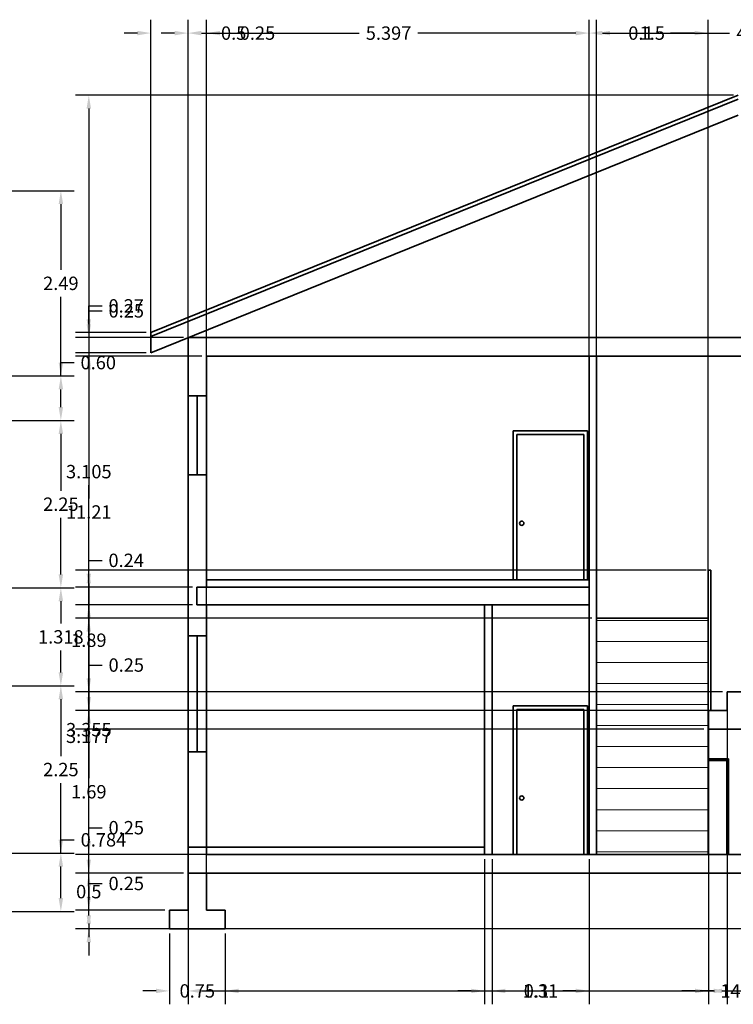
# Model space of a CAD drawing. Units: metres. Extents: x 14054 to 28215, y 4175 to 8383.
# Tile 5 of 6: x 14096.96 to 14106.56, y 4179.48 to 4192.72. Entities that reach past the tile are written whole.
import ezdxf

# ---------------------------------------------------------------- set-up
doc = ezdxf.new("R2010")
doc.units = ezdxf.units.M
for name, color, linetype, lineweight in [('A-ANNO-DIMS', 2, 'Continuous', 18), ('A-ANNO-NPLT', 9, 'Continuous', 13), ('A-SECT', 1, 'Continuous', 35), ('A-WALL-PATT', 8, 'Continuous', 13)]:
    doc.layers.add(name, color=color, linetype=linetype, lineweight=lineweight)
doc.styles.get("Standard").update_dxf_attribs({"font": 'arial.ttf'})
doc.dimstyles.get("Standard").update_dxf_attribs({"dimtxt": 0.18, "dimasz": 0.18, "dimexe": 0.18, "dimexo": 0.0625, "dimgap": 0.09, "dimtad": 0, "dimtih": 1, "dimtoh": 1, "dimdec": 4, "dimzin": 0, "dimdsep": 46, "dimtxsty": 'Standard', "dimcen": 0.09, "dimadec": 0, "dimazin": 0, "dimtfac": 1, "dimtdec": 4, "dimtofl": 0, "dimtmove": 0, "dimatfit": 3, "dimfxl": 1, "dimtolj": 1, "dimtzin": 0, "dimarcsym": 0})

# ---------------------------------------------------------------- blocks, each defined once
blk = doc.blocks.new('*D23')
at = {"layer": 'A-ANNO-DIMS', "color": 0, "lineweight": -2, "transparency": 16777216}
for p, q in [((14097.511, 4181.511), (14097.511, 4181.691)), ((14097.511, 4181.691), (14097.691, 4181.691)), ((14092.904, 4181.511), (14097.691, 4181.511)), ((14097.511, 4180.908), (14097.511, 4181.331)), ((14094.951, 4180.728), (14097.691, 4180.728))]:
    blk.add_line(p, q, dxfattribs=at)
at = {"layer": 'A-ANNO-DIMS', "color": 0, "transparency": 16777216}
for points in [[(14097.481, 4181.331), (14097.541, 4181.331), (14097.511, 4181.511)], [(14097.481, 4180.908), (14097.541, 4180.908), (14097.511, 4180.728)]]:
    blk.add_solid(points, dxfattribs=at)
at = {"layer": 'Defpoints', "color": 0, "transparency": 16777216}
for p in [(14092.842, 4181.511), (14097.511, 4181.511), (14094.888, 4180.728)]:
    blk.add_point(p, dxfattribs=at)
at = {"layer": 'A-ANNO-DIMS', "color": 0, "transparency": 16777216, "insert": (14098.084, 4181.691), "char_height": 0.18, "attachment_point": 5}
blk.add_mtext('\\A1;0.784', dxfattribs=at)
blk = doc.blocks.new('*D24')
at = {"layer": 'A-ANNO-DIMS', "color": 0, "lineweight": -2, "transparency": 16777216}
for p, q in [((14092.904, 4183.761), (14097.691, 4183.761)), ((14097.511, 4183.581), (14097.511, 4182.818)), ((14097.511, 4181.691), (14097.511, 4182.454)), ((14092.904, 4181.511), (14097.691, 4181.511))]:
    blk.add_line(p, q, dxfattribs=at)
at = {"layer": 'A-ANNO-DIMS', "color": 0, "transparency": 16777216}
for points in [[(14097.481, 4183.581), (14097.541, 4183.581), (14097.511, 4183.761)], [(14097.481, 4181.691), (14097.541, 4181.691), (14097.511, 4181.511)]]:
    blk.add_solid(points, dxfattribs=at)
at = {"layer": 'Defpoints', "color": 0, "transparency": 16777216}
for p in [(14092.842, 4183.761), (14097.511, 4183.761), (14092.842, 4181.511)]:
    blk.add_point(p, dxfattribs=at)
at = {"layer": 'A-ANNO-DIMS', "color": 0, "transparency": 16777216, "insert": (14097.511, 4182.636), "char_height": 0.18, "attachment_point": 5}
blk.add_mtext('\\A1;2.25', dxfattribs=at)
blk = doc.blocks.new('*D25')
at = {"layer": 'A-ANNO-DIMS', "color": 0, "lineweight": -2, "transparency": 16777216}
for p, q in [((14092.904, 4185.079), (14097.691, 4185.079)), ((14097.511, 4184.899), (14097.511, 4184.602)), ((14097.511, 4183.941), (14097.511, 4184.238)), ((14092.904, 4183.761), (14097.691, 4183.761))]:
    blk.add_line(p, q, dxfattribs=at)
at = {"layer": 'A-ANNO-DIMS', "color": 0, "transparency": 16777216}
for points in [[(14097.481, 4184.899), (14097.541, 4184.899), (14097.511, 4185.079)], [(14097.481, 4183.941), (14097.541, 4183.941), (14097.511, 4183.761)]]:
    blk.add_solid(points, dxfattribs=at)
at = {"layer": 'Defpoints', "color": 0, "transparency": 16777216}
for p in [(14092.842, 4185.079), (14097.511, 4185.079), (14092.842, 4183.761)]:
    blk.add_point(p, dxfattribs=at)
at = {"layer": 'A-ANNO-DIMS', "color": 0, "transparency": 16777216, "insert": (14097.511, 4184.42), "char_height": 0.18, "attachment_point": 5}
blk.add_mtext('\\A1;1.318', dxfattribs=at)
blk = doc.blocks.new('*D26')
at = {"layer": 'A-ANNO-DIMS', "color": 0, "lineweight": -2, "transparency": 16777216}
for p, q in [((14092.904, 4187.329), (14097.691, 4187.329)), ((14097.511, 4187.149), (14097.511, 4186.386)), ((14097.511, 4185.259), (14097.511, 4186.022)), ((14092.904, 4185.079), (14097.691, 4185.079))]:
    blk.add_line(p, q, dxfattribs=at)
at = {"layer": 'A-ANNO-DIMS', "color": 0, "transparency": 16777216}
for points in [[(14097.481, 4187.149), (14097.541, 4187.149), (14097.511, 4187.329)], [(14097.481, 4185.259), (14097.541, 4185.259), (14097.511, 4185.079)]]:
    blk.add_solid(points, dxfattribs=at)
at = {"layer": 'Defpoints', "color": 0, "transparency": 16777216}
for p in [(14092.842, 4187.329), (14097.511, 4187.329), (14092.842, 4185.079)]:
    blk.add_point(p, dxfattribs=at)
at = {"layer": 'A-ANNO-DIMS', "color": 0, "transparency": 16777216, "insert": (14097.511, 4186.204), "char_height": 0.18, "attachment_point": 5}
blk.add_mtext('\\A1;2.25', dxfattribs=at)
blk = doc.blocks.new('*D27')
at = {"layer": 'A-ANNO-DIMS', "color": 0, "lineweight": -2, "transparency": 16777216}
for p, q in [((14097.511, 4187.928), (14097.511, 4188.108)), ((14097.511, 4188.108), (14097.691, 4188.108)), ((14096.633, 4187.928), (14097.691, 4187.928)), ((14097.511, 4187.509), (14097.511, 4187.748)), ((14092.904, 4187.329), (14097.691, 4187.329))]:
    blk.add_line(p, q, dxfattribs=at)
at = {"layer": 'A-ANNO-DIMS', "color": 0, "transparency": 16777216}
for points in [[(14097.481, 4187.748), (14097.541, 4187.748), (14097.511, 4187.928)], [(14097.481, 4187.509), (14097.541, 4187.509), (14097.511, 4187.329)]]:
    blk.add_solid(points, dxfattribs=at)
at = {"layer": 'Defpoints', "color": 0, "transparency": 16777216}
for p in [(14096.571, 4187.928), (14097.511, 4187.928), (14092.842, 4187.329)]:
    blk.add_point(p, dxfattribs=at)
at = {"layer": 'A-ANNO-DIMS', "color": 0, "transparency": 16777216, "insert": (14098.014, 4188.108), "char_height": 0.18, "attachment_point": 5}
blk.add_mtext('\\A1;0.60', dxfattribs=at)
blk = doc.blocks.new('*D28')
at = {"layer": 'A-ANNO-DIMS', "color": 0, "lineweight": -2, "transparency": 16777216}
for p, q in [((14087.501, 4190.42), (14097.691, 4190.42)), ((14097.511, 4190.24), (14097.511, 4189.356)), ((14097.511, 4188.108), (14097.511, 4188.992)), ((14096.633, 4187.928), (14097.691, 4187.928))]:
    blk.add_line(p, q, dxfattribs=at)
at = {"layer": 'A-ANNO-DIMS', "color": 0, "transparency": 16777216}
for points in [[(14097.481, 4190.24), (14097.541, 4190.24), (14097.511, 4190.42)], [(14097.481, 4188.108), (14097.541, 4188.108), (14097.511, 4187.928)]]:
    blk.add_solid(points, dxfattribs=at)
at = {"layer": 'Defpoints', "color": 0, "transparency": 16777216}
for p in [(14087.438, 4190.42), (14097.511, 4190.42), (14096.571, 4187.928)]:
    blk.add_point(p, dxfattribs=at)
at = {"layer": 'A-ANNO-DIMS', "color": 0, "transparency": 16777216, "insert": (14097.511, 4189.174), "char_height": 0.18, "attachment_point": 5}
blk.add_mtext('\\A1;2.49', dxfattribs=at)
blk = doc.blocks.new('*D29')
at = {"layer": 'A-ANNO-DIMS', "color": 0, "lineweight": -2, "transparency": 16777216}
for p, q in [((14098.722, 4188.304), (14098.722, 4192.719)), ((14099.222, 4188.507), (14099.222, 4192.719)), ((14098.542, 4192.539), (14098.362, 4192.539)), ((14099.402, 4192.539), (14099.582, 4192.539))]:
    blk.add_line(p, q, dxfattribs=at)
at = {"layer": 'A-ANNO-DIMS', "color": 0, "transparency": 16777216}
for points in [[(14098.542, 4192.569), (14098.542, 4192.509), (14098.722, 4192.539)], [(14099.402, 4192.569), (14099.402, 4192.509), (14099.222, 4192.539)]]:
    blk.add_solid(points, dxfattribs=at)
at = {"layer": 'Defpoints', "color": 0, "transparency": 16777216}
for p in [(14099.222, 4192.539), (14099.222, 4188.444), (14098.722, 4188.241)]:
    blk.add_point(p, dxfattribs=at)
at = {"layer": 'A-ANNO-DIMS', "color": 0, "transparency": 16777216, "insert": (14099.836, 4192.539), "char_height": 0.18, "attachment_point": 5}
blk.add_mtext('\\A1;0.5', dxfattribs=at)
blk = doc.blocks.new('*D30')
at = {"layer": 'A-ANNO-DIMS', "color": 0, "lineweight": -2, "transparency": 16777216}
for p, q in [((14099.222, 4188.507), (14099.222, 4192.719)), ((14104.618, 4188.257), (14104.618, 4192.719)), ((14099.402, 4192.539), (14101.526, 4192.539)), ((14104.438, 4192.539), (14102.314, 4192.539))]:
    blk.add_line(p, q, dxfattribs=at)
at = {"layer": 'A-ANNO-DIMS', "color": 0, "transparency": 16777216}
for points in [[(14099.402, 4192.569), (14099.402, 4192.509), (14099.222, 4192.539)], [(14104.438, 4192.569), (14104.438, 4192.509), (14104.618, 4192.539)]]:
    blk.add_solid(points, dxfattribs=at)
at = {"layer": 'Defpoints', "color": 0, "transparency": 16777216}
for p in [(14104.618, 4192.539), (14099.222, 4188.444), (14104.618, 4188.194)]:
    blk.add_point(p, dxfattribs=at)
at = {"layer": 'A-ANNO-DIMS', "color": 0, "transparency": 16777216, "insert": (14101.92, 4192.539), "char_height": 0.18, "attachment_point": 5}
blk.add_mtext('\\A1;5.397', dxfattribs=at)
blk = doc.blocks.new('*D31')
at = {"layer": 'A-ANNO-DIMS', "color": 0, "lineweight": -2, "transparency": 16777216}
for p, q in [((14104.618, 4188.257), (14104.618, 4192.719)), ((14109.195, 4188.257), (14109.195, 4192.719)), ((14104.798, 4192.539), (14106.509, 4192.539)), ((14109.015, 4192.539), (14107.304, 4192.539))]:
    blk.add_line(p, q, dxfattribs=at)
at = {"layer": 'A-ANNO-DIMS', "color": 0, "transparency": 16777216}
for points in [[(14104.798, 4192.569), (14104.798, 4192.509), (14104.618, 4192.539)], [(14109.015, 4192.569), (14109.015, 4192.509), (14109.195, 4192.539)]]:
    blk.add_solid(points, dxfattribs=at)
at = {"layer": 'Defpoints', "color": 0, "transparency": 16777216}
for p in [(14109.195, 4192.539), (14104.618, 4188.194), (14109.195, 4188.194)]:
    blk.add_point(p, dxfattribs=at)
at = {"layer": 'A-ANNO-DIMS', "color": 0, "transparency": 16777216, "insert": (14106.907, 4192.539), "char_height": 0.18, "attachment_point": 5}
blk.add_mtext('\\A1;4.577', dxfattribs=at)
blk = doc.blocks.new('*D34')
at = {"layer": 'A-ANNO-DIMS', "color": 0, "lineweight": -2, "transparency": 16777216}
for p, q in [((14099.222, 4181.182), (14099.222, 4179.479)), ((14114.022, 4181.182), (14114.022, 4179.479)), ((14099.402, 4179.659), (14106.306, 4179.659)), ((14113.842, 4179.659), (14106.937, 4179.659))]:
    blk.add_line(p, q, dxfattribs=at)
at = {"layer": 'A-ANNO-DIMS', "color": 0, "transparency": 16777216}
for points in [[(14099.402, 4179.689), (14099.402, 4179.629), (14099.222, 4179.659)], [(14113.842, 4179.689), (14113.842, 4179.629), (14114.022, 4179.659)]]:
    blk.add_solid(points, dxfattribs=at)
at = {"layer": 'Defpoints', "color": 0, "transparency": 16777216}
for p in [(14099.222, 4181.244), (14114.022, 4181.244), (14114.022, 4179.659)]:
    blk.add_point(p, dxfattribs=at)
at = {"layer": 'A-ANNO-DIMS', "color": 0, "transparency": 16777216, "insert": (14106.622, 4179.659), "char_height": 0.18, "attachment_point": 5}
blk.add_mtext('\\A1;14.8', dxfattribs=at)
blk = doc.blocks.new('*D39')
at = {"layer": 'A-ANNO-DIMS', "color": 0, "lineweight": -2, "transparency": 16777216}
for p, q in [((14106.559, 4191.704), (14097.707, 4191.704)), ((14097.887, 4191.524), (14097.887, 4186.28)), ((14097.887, 4180.674), (14097.887, 4185.919)), ((14114.209, 4180.494), (14097.707, 4180.494))]:
    blk.add_line(p, q, dxfattribs=at)
at = {"layer": 'A-ANNO-DIMS', "color": 0, "transparency": 16777216}
for points in [[(14097.857, 4191.524), (14097.917, 4191.524), (14097.887, 4191.704)], [(14097.857, 4180.674), (14097.917, 4180.674), (14097.887, 4180.494)]]:
    blk.add_solid(points, dxfattribs=at)
at = {"layer": 'Defpoints', "color": 0, "transparency": 16777216}
for p in [(14097.887, 4191.704), (14106.622, 4191.704), (14114.272, 4180.494)]:
    blk.add_point(p, dxfattribs=at)
at = {"layer": 'A-ANNO-DIMS', "color": 0, "transparency": 16777216, "insert": (14097.887, 4186.099), "char_height": 0.18, "attachment_point": 5}
blk.add_mtext('\\A1;11.21', dxfattribs=at)
blk = doc.blocks.new('*D45')
at = {"layer": 'A-ANNO-DIMS', "color": 0, "lineweight": -2, "transparency": 16777216}
for p, q in [((14097.887, 4180.924), (14097.887, 4181.104)), ((14097.887, 4181.104), (14098.067, 4181.104)), ((14098.909, 4180.744), (14097.707, 4180.744)), ((14098.909, 4180.494), (14097.707, 4180.494)), ((14097.887, 4180.314), (14097.887, 4180.134))]:
    blk.add_line(p, q, dxfattribs=at)
at = {"layer": 'A-ANNO-DIMS', "color": 0, "transparency": 16777216}
for points in [[(14097.857, 4180.924), (14097.917, 4180.924), (14097.887, 4180.744)], [(14097.857, 4180.314), (14097.917, 4180.314), (14097.887, 4180.494)]]:
    blk.add_solid(points, dxfattribs=at)
at = {"layer": 'Defpoints', "color": 0, "transparency": 16777216}
for p in [(14097.887, 4180.744), (14098.972, 4180.744), (14098.972, 4180.494)]:
    blk.add_point(p, dxfattribs=at)
at = {"layer": 'A-ANNO-DIMS', "color": 0, "transparency": 16777216, "insert": (14098.391, 4181.104), "char_height": 0.18, "attachment_point": 5}
blk.add_mtext('\\A1;0.25', dxfattribs=at)
blk = doc.blocks.new('*D46')
at = {"layer": 'A-ANNO-DIMS', "color": 0, "lineweight": -2, "transparency": 16777216}
for p, q in [((14097.886638, 4181.424065), (14097.886638, 4181.604065)), ((14099.159089, 4181.244065), (14097.706638, 4181.244065)), ((14098.909089, 4180.744065), (14097.706638, 4180.744065)), ((14097.886638, 4180.564065), (14097.886638, 4180.384065))]:
    blk.add_line(p, q, dxfattribs=at)
at = {"layer": 'A-ANNO-DIMS', "color": 0, "transparency": 16777216}
for points in [[(14097.856638, 4181.424065), (14097.916638, 4181.424065), (14097.886638, 4181.244065)], [(14097.856638, 4180.564065), (14097.916638, 4180.564065), (14097.886638, 4180.744065)]]:
    blk.add_solid(points, dxfattribs=at)
at = {"layer": 'Defpoints', "color": 0, "transparency": 16777216}
for p in [(14097.886638, 4181.244065), (14099.221589, 4181.244065), (14098.971589, 4180.744065)]:
    blk.add_point(p, dxfattribs=at)
at = {"layer": 'A-ANNO-DIMS', "color": 0, "transparency": 16777216, "insert": (14097.886638, 4180.994065), "char_height": 0.18, "attachment_point": 5}
blk.add_mtext('\\A1;0.5', dxfattribs=at)
blk = doc.blocks.new('*D47')
at = {"layer": 'A-ANNO-DIMS', "color": 0, "lineweight": -2, "transparency": 16777216}
for p, q in [((14097.887, 4181.674), (14097.887, 4181.854)), ((14097.887, 4181.854), (14098.067, 4181.854)), ((14099.409, 4181.494), (14097.707, 4181.494)), ((14099.159, 4181.244), (14097.707, 4181.244)), ((14097.887, 4181.064), (14097.887, 4180.884))]:
    blk.add_line(p, q, dxfattribs=at)
at = {"layer": 'A-ANNO-DIMS', "color": 0, "transparency": 16777216}
for points in [[(14097.857, 4181.674), (14097.917, 4181.674), (14097.887, 4181.494)], [(14097.857, 4181.064), (14097.917, 4181.064), (14097.887, 4181.244)]]:
    blk.add_solid(points, dxfattribs=at)
at = {"layer": 'Defpoints', "color": 0, "transparency": 16777216}
for p in [(14097.887, 4181.494), (14099.472, 4181.494), (14099.222, 4181.244)]:
    blk.add_point(p, dxfattribs=at)
at = {"layer": 'A-ANNO-DIMS', "color": 0, "transparency": 16777216, "insert": (14098.391, 4181.854), "char_height": 0.18, "attachment_point": 5}
blk.add_mtext('\\A1;0.25', dxfattribs=at)
blk = doc.blocks.new('*D48')
at = {"layer": 'A-ANNO-DIMS', "color": 0, "lineweight": -2, "transparency": 16777216}
for p, q in [((14099.222, 4180.807), (14099.222, 4192.719)), ((14099.472, 4180.807), (14099.472, 4192.719)), ((14099.042, 4192.539), (14098.862, 4192.539)), ((14099.652, 4192.539), (14099.832, 4192.539))]:
    blk.add_line(p, q, dxfattribs=at)
at = {"layer": 'A-ANNO-DIMS', "color": 0, "transparency": 16777216}
for points in [[(14099.042, 4192.569), (14099.042, 4192.509), (14099.222, 4192.539)], [(14099.652, 4192.569), (14099.652, 4192.509), (14099.472, 4192.539)]]:
    blk.add_solid(points, dxfattribs=at)
at = {"layer": 'Defpoints', "color": 0, "transparency": 16777216}
for p in [(14099.472, 4192.539), (14099.222, 4180.744), (14099.472, 4180.744)]:
    blk.add_point(p, dxfattribs=at)
at = {"layer": 'A-ANNO-DIMS', "color": 0, "transparency": 16777216, "insert": (14100.156, 4192.539), "char_height": 0.18, "attachment_point": 5}
blk.add_mtext('\\A1;0.25', dxfattribs=at)
blk = doc.blocks.new('*D49')
at = {"layer": 'A-ANNO-DIMS', "color": 0, "lineweight": -2, "transparency": 16777216}
for p, q in [((14098.971589, 4180.431565), (14098.971589, 4179.479065)), ((14099.721589, 4180.431565), (14099.721589, 4179.479065)), ((14098.791589, 4179.659065), (14098.611589, 4179.659065)), ((14099.901589, 4179.659065), (14100.081589, 4179.659065))]:
    blk.add_line(p, q, dxfattribs=at)
at = {"layer": 'A-ANNO-DIMS', "color": 0, "transparency": 16777216}
for points in [[(14098.791589, 4179.689065), (14098.791589, 4179.629065), (14098.971589, 4179.659065)], [(14099.901589, 4179.689065), (14099.901589, 4179.629065), (14099.721589, 4179.659065)]]:
    blk.add_solid(points, dxfattribs=at)
at = {"layer": 'Defpoints', "color": 0, "transparency": 16777216}
for p in [(14098.971589, 4180.494065), (14099.721589, 4180.494065), (14099.721589, 4179.659065)]:
    blk.add_point(p, dxfattribs=at)
at = {"layer": 'A-ANNO-DIMS', "color": 0, "transparency": 16777216, "insert": (14099.346589, 4179.659065), "char_height": 0.18, "attachment_point": 5}
blk.add_mtext('\\A1;0.75', dxfattribs=at)
blk = doc.blocks.new('*D50')
at = {"layer": 'A-ANNO-DIMS', "color": 0, "lineweight": -2, "transparency": 16777216}
for p, q in [((14099.28, 4184.849), (14097.707, 4184.849)), ((14097.887, 4184.669), (14097.887, 4183.354)), ((14097.887, 4181.674), (14097.887, 4182.99)), ((14099.409, 4181.494), (14097.707, 4181.494))]:
    blk.add_line(p, q, dxfattribs=at)
at = {"layer": 'A-ANNO-DIMS', "color": 0, "transparency": 16777216}
for points in [[(14097.857, 4184.669), (14097.917, 4184.669), (14097.887, 4184.849)], [(14097.857, 4181.674), (14097.917, 4181.674), (14097.887, 4181.494)]]:
    blk.add_solid(points, dxfattribs=at)
at = {"layer": 'Defpoints', "color": 0, "transparency": 16777216}
for p in [(14097.887, 4184.849), (14099.342, 4184.849), (14099.472, 4181.494)]:
    blk.add_point(p, dxfattribs=at)
at = {"layer": 'A-ANNO-DIMS', "color": 0, "transparency": 16777216, "insert": (14097.887, 4183.172), "char_height": 0.18, "attachment_point": 5}
blk.add_mtext('\\A1;3.355', dxfattribs=at)
blk = doc.blocks.new('*D51')
at = {"layer": 'A-ANNO-DIMS', "color": 0, "lineweight": -2, "transparency": 16777216}
for p, q in [((14097.887, 4185.269), (14097.887, 4185.449)), ((14097.887, 4185.449), (14098.067, 4185.449)), ((14099.28, 4185.089), (14097.707, 4185.089)), ((14099.28, 4184.849), (14097.707, 4184.849)), ((14097.887, 4184.669), (14097.887, 4184.489))]:
    blk.add_line(p, q, dxfattribs=at)
at = {"layer": 'A-ANNO-DIMS', "color": 0, "transparency": 16777216}
for points in [[(14097.857, 4185.269), (14097.917, 4185.269), (14097.887, 4185.089)], [(14097.857, 4184.669), (14097.917, 4184.669), (14097.887, 4184.849)]]:
    blk.add_solid(points, dxfattribs=at)
at = {"layer": 'Defpoints', "color": 0, "transparency": 16777216}
for p in [(14097.887, 4185.089), (14099.342, 4185.089), (14099.342, 4184.849)]:
    blk.add_point(p, dxfattribs=at)
at = {"layer": 'A-ANNO-DIMS', "color": 0, "transparency": 16777216, "insert": (14098.39, 4185.449), "char_height": 0.18, "attachment_point": 5}
blk.add_mtext('\\A1;0.24', dxfattribs=at)
blk = doc.blocks.new('*D52')
at = {"layer": 'A-ANNO-DIMS', "color": 0, "lineweight": -2, "transparency": 16777216}
for p, q in [((14099.409, 4188.194), (14097.707, 4188.194)), ((14097.887, 4188.014), (14097.887, 4186.824)), ((14097.887, 4185.269), (14097.887, 4186.46)), ((14099.28, 4185.089), (14097.707, 4185.089))]:
    blk.add_line(p, q, dxfattribs=at)
at = {"layer": 'A-ANNO-DIMS', "color": 0, "transparency": 16777216}
for points in [[(14097.857, 4188.014), (14097.917, 4188.014), (14097.887, 4188.194)], [(14097.857, 4185.269), (14097.917, 4185.269), (14097.887, 4185.089)]]:
    blk.add_solid(points, dxfattribs=at)
at = {"layer": 'Defpoints', "color": 0, "transparency": 16777216}
for p in [(14097.887, 4188.194), (14099.472, 4188.194), (14099.342, 4185.089)]:
    blk.add_point(p, dxfattribs=at)
at = {"layer": 'A-ANNO-DIMS', "color": 0, "transparency": 16777216, "insert": (14097.887, 4186.642), "char_height": 0.18, "attachment_point": 5}
blk.add_mtext('\\A1;3.105', dxfattribs=at)
blk = doc.blocks.new('*D53')
at = {"layer": 'A-ANNO-DIMS', "color": 0, "lineweight": -2, "transparency": 16777216}
for p, q in [((14097.887, 4188.624), (14097.887, 4188.804)), ((14097.887, 4188.804), (14098.067, 4188.804)), ((14099.159, 4188.444), (14097.707, 4188.444)), ((14099.409, 4188.194), (14097.707, 4188.194)), ((14097.887, 4188.014), (14097.887, 4187.834))]:
    blk.add_line(p, q, dxfattribs=at)
at = {"layer": 'A-ANNO-DIMS', "color": 0, "transparency": 16777216}
for points in [[(14097.857, 4188.624), (14097.917, 4188.624), (14097.887, 4188.444)], [(14097.857, 4188.014), (14097.917, 4188.014), (14097.887, 4188.194)]]:
    blk.add_solid(points, dxfattribs=at)
at = {"layer": 'Defpoints', "color": 0, "transparency": 16777216}
for p in [(14097.887, 4188.444), (14099.222, 4188.444), (14099.472, 4188.194)]:
    blk.add_point(p, dxfattribs=at)
at = {"layer": 'A-ANNO-DIMS', "color": 0, "transparency": 16777216, "insert": (14098.391, 4188.804), "char_height": 0.18, "attachment_point": 5}
blk.add_mtext('\\A1;0.25', dxfattribs=at)
blk = doc.blocks.new('*D54')
at = {"layer": 'A-ANNO-DIMS', "color": 0, "lineweight": -2, "transparency": 16777216}
for p, q in [((14097.886638, 4188.691044), (14097.886638, 4188.871044)), ((14097.886638, 4188.871044), (14098.066638, 4188.871044)), ((14098.659138, 4188.511044), (14097.706638, 4188.511044)), ((14098.659138, 4188.241394), (14097.706638, 4188.241394)), ((14097.886638, 4188.061394), (14097.886638, 4187.881394))]:
    blk.add_line(p, q, dxfattribs=at)
at = {"layer": 'A-ANNO-DIMS', "color": 0, "transparency": 16777216}
for points in [[(14097.856638, 4188.691044), (14097.916638, 4188.691044), (14097.886638, 4188.511044)], [(14097.856638, 4188.061394), (14097.916638, 4188.061394), (14097.886638, 4188.241394)]]:
    blk.add_solid(points, dxfattribs=at)
at = {"layer": 'Defpoints', "color": 0, "transparency": 16777216}
for p in [(14097.886638, 4188.511044), (14098.721638, 4188.511044), (14098.721638, 4188.241394)]:
    blk.add_point(p, dxfattribs=at)
at = {"layer": 'A-ANNO-DIMS', "color": 0, "transparency": 16777216, "insert": (14098.390417, 4188.871044), "char_height": 0.18, "attachment_point": 5}
blk.add_mtext('\\A1;0.27', dxfattribs=at)
blk = doc.blocks.new('*D55')
at = {"layer": 'A-ANNO-DIMS', "color": 0, "lineweight": -2, "transparency": 16777216}
for p, q in [((14103.212, 4181.432), (14103.212, 4179.479)), ((14103.312, 4181.432), (14103.312, 4179.479)), ((14103.032, 4179.659), (14102.852, 4179.659)), ((14103.492, 4179.659), (14103.672, 4179.659))]:
    blk.add_line(p, q, dxfattribs=at)
at = {"layer": 'A-ANNO-DIMS', "color": 0, "transparency": 16777216}
for points in [[(14103.032, 4179.689), (14103.032, 4179.629), (14103.212, 4179.659)], [(14103.492, 4179.689), (14103.492, 4179.629), (14103.312, 4179.659)]]:
    blk.add_solid(points, dxfattribs=at)
at = {"layer": 'Defpoints', "color": 0, "transparency": 16777216}
for p in [(14103.212, 4181.494), (14103.312, 4181.494), (14103.312, 4179.659)]:
    blk.add_point(p, dxfattribs=at)
at = {"layer": 'A-ANNO-DIMS', "color": 0, "transparency": 16777216, "insert": (14103.909, 4179.659), "char_height": 0.18, "attachment_point": 5}
blk.add_mtext('\\A1;0.1', dxfattribs=at)
blk = doc.blocks.new('*D56')
at = {"layer": 'A-ANNO-DIMS', "color": 0, "lineweight": -2, "transparency": 16777216}
for p, q in [((14103.312, 4181.432), (14103.312, 4179.479)), ((14104.618, 4181.432), (14104.618, 4179.479)), ((14103.492, 4179.659), (14103.667, 4179.659)), ((14104.438, 4179.659), (14104.263, 4179.659))]:
    blk.add_line(p, q, dxfattribs=at)
at = {"layer": 'A-ANNO-DIMS', "color": 0, "transparency": 16777216}
for points in [[(14103.492, 4179.689), (14103.492, 4179.629), (14103.312, 4179.659)], [(14104.438, 4179.689), (14104.438, 4179.629), (14104.618, 4179.659)]]:
    blk.add_solid(points, dxfattribs=at)
at = {"layer": 'Defpoints', "color": 0, "transparency": 16777216}
for p in [(14103.312, 4181.494), (14104.618, 4181.494), (14104.618, 4179.659)]:
    blk.add_point(p, dxfattribs=at)
at = {"layer": 'A-ANNO-DIMS', "color": 0, "transparency": 16777216, "insert": (14103.965, 4179.659), "char_height": 0.18, "attachment_point": 5}
blk.add_mtext('\\A1;1.31', dxfattribs=at)
blk = doc.blocks.new('*D57')
at = {"layer": 'A-ANNO-DIMS', "color": 0, "lineweight": -2, "transparency": 16777216}
for p, q in [((14104.618, 4184.912), (14104.618, 4192.719)), ((14104.718, 4184.733), (14104.718, 4192.719)), ((14104.438, 4192.539), (14104.258, 4192.539)), ((14104.898, 4192.539), (14105.078, 4192.539))]:
    blk.add_line(p, q, dxfattribs=at)
at = {"layer": 'A-ANNO-DIMS', "color": 0, "transparency": 16777216}
for points in [[(14104.438, 4192.569), (14104.438, 4192.509), (14104.618, 4192.539)], [(14104.898, 4192.569), (14104.898, 4192.509), (14104.718, 4192.539)]]:
    blk.add_solid(points, dxfattribs=at)
at = {"layer": 'Defpoints', "color": 0, "transparency": 16777216}
for p in [(14104.718, 4192.539), (14104.618, 4184.849), (14104.718, 4184.671)]:
    blk.add_point(p, dxfattribs=at)
at = {"layer": 'A-ANNO-DIMS', "color": 0, "transparency": 16777216, "insert": (14105.315, 4192.539), "char_height": 0.18, "attachment_point": 5}
blk.add_mtext('\\A1;0.1', dxfattribs=at)
blk = doc.blocks.new('*D58')
at = {"layer": 'A-ANNO-DIMS', "color": 0, "lineweight": -2, "transparency": 16777216}
for p, q in [((14104.718, 4184.733), (14104.718, 4192.719)), ((14106.218, 4184.733), (14106.218, 4192.719)), ((14104.898, 4192.539), (14105.222, 4192.539)), ((14106.038, 4192.539), (14105.714, 4192.539))]:
    blk.add_line(p, q, dxfattribs=at)
at = {"layer": 'A-ANNO-DIMS', "color": 0, "transparency": 16777216}
for points in [[(14104.898, 4192.569), (14104.898, 4192.509), (14104.718, 4192.539)], [(14106.038, 4192.569), (14106.038, 4192.509), (14106.218, 4192.539)]]:
    blk.add_solid(points, dxfattribs=at)
at = {"layer": 'Defpoints', "color": 0, "transparency": 16777216}
for p in [(14106.218, 4192.539), (14104.718, 4184.671), (14106.218, 4184.671)]:
    blk.add_point(p, dxfattribs=at)
at = {"layer": 'A-ANNO-DIMS', "color": 0, "transparency": 16777216, "insert": (14105.468, 4192.539), "char_height": 0.18, "attachment_point": 5}
blk.add_mtext('\\A1;1.5', dxfattribs=at)
blk = doc.blocks.new('*D59')
at = {"layer": 'A-ANNO-DIMS', "color": 0, "lineweight": -2, "transparency": 16777216}
for p, q in [((14104.656, 4184.671), (14097.707, 4184.671)), ((14097.887, 4184.491), (14097.887, 4183.264)), ((14097.887, 4181.674), (14097.887, 4182.901)), ((14104.656, 4181.494), (14097.707, 4181.494))]:
    blk.add_line(p, q, dxfattribs=at)
at = {"layer": 'A-ANNO-DIMS', "color": 0, "transparency": 16777216}
for points in [[(14097.857, 4184.491), (14097.917, 4184.491), (14097.887, 4184.671)], [(14097.857, 4181.674), (14097.917, 4181.674), (14097.887, 4181.494)]]:
    blk.add_solid(points, dxfattribs=at)
at = {"layer": 'Defpoints', "color": 0, "transparency": 16777216}
for p in [(14097.887, 4184.671), (14104.718, 4184.671), (14104.718, 4181.494)]:
    blk.add_point(p, dxfattribs=at)
at = {"layer": 'A-ANNO-DIMS', "color": 0, "transparency": 16777216, "insert": (14097.887, 4183.083), "char_height": 0.18, "attachment_point": 5}
blk.add_mtext('\\A1;3.177', dxfattribs=at)
blk = doc.blocks.new('*D60')
at = {"layer": 'A-ANNO-DIMS', "color": 0, "lineweight": -2, "transparency": 16777216}
for p, q in [((14107.951, 4184.863), (14107.951, 4179.479)), ((14106.224, 4183.368), (14106.224, 4179.479)), ((14106.404, 4179.659), (14106.772, 4179.659)), ((14107.771, 4179.659), (14107.403, 4179.659))]:
    blk.add_line(p, q, dxfattribs=at)
at = {"layer": 'A-ANNO-DIMS', "color": 0, "transparency": 16777216}
for points in [[(14106.404, 4179.689), (14106.404, 4179.629), (14106.224, 4179.659)], [(14107.771, 4179.689), (14107.771, 4179.629), (14107.951, 4179.659)]]:
    blk.add_solid(points, dxfattribs=at)
at = {"layer": 'Defpoints', "color": 0, "transparency": 16777216}
for p in [(14107.951, 4184.925), (14106.224, 4183.431), (14107.951, 4179.659)]:
    blk.add_point(p, dxfattribs=at)
at = {"layer": 'A-ANNO-DIMS', "color": 0, "transparency": 16777216, "insert": (14107.088, 4179.659), "char_height": 0.18, "attachment_point": 5}
blk.add_mtext('\\A1;1.73', dxfattribs=at)
blk = doc.blocks.new('*D61')
at = {"layer": 'A-ANNO-DIMS', "color": 0, "lineweight": -2, "transparency": 16777216}
for p, q in [((14097.887, 4183.861), (14097.887, 4184.041)), ((14097.887, 4184.041), (14098.067, 4184.041)), ((14106.411, 4183.681), (14097.707, 4183.681)), ((14106.411, 4183.431), (14097.707, 4183.431)), ((14097.887, 4183.251), (14097.887, 4183.071))]:
    blk.add_line(p, q, dxfattribs=at)
at = {"layer": 'A-ANNO-DIMS', "color": 0, "transparency": 16777216}
for points in [[(14097.857, 4183.861), (14097.917, 4183.861), (14097.887, 4183.681)], [(14097.857, 4183.251), (14097.917, 4183.251), (14097.887, 4183.431)]]:
    blk.add_solid(points, dxfattribs=at)
at = {"layer": 'Defpoints', "color": 0, "transparency": 16777216}
for p in [(14097.887, 4183.681), (14106.474, 4183.681), (14106.474, 4183.431)]:
    blk.add_point(p, dxfattribs=at)
at = {"layer": 'A-ANNO-DIMS', "color": 0, "transparency": 16777216, "insert": (14098.391, 4184.041), "char_height": 0.18, "attachment_point": 5}
blk.add_mtext('\\A1;0.25', dxfattribs=at)
blk = doc.blocks.new('*D62')
at = {"layer": 'A-ANNO-DIMS', "color": 0, "lineweight": -2, "transparency": 16777216}
for p, q in [((14106.473765, 4183.618165), (14106.473765, 4179.479065)), ((14106.701342, 4183.618165), (14106.701342, 4179.479065)), ((14106.293765, 4179.659065), (14106.113765, 4179.659065)), ((14106.881342, 4179.659065), (14107.061342, 4179.659065))]:
    blk.add_line(p, q, dxfattribs=at)
at = {"layer": 'A-ANNO-DIMS', "color": 0, "transparency": 16777216}
for points in [[(14106.293765, 4179.689065), (14106.293765, 4179.629065), (14106.473765, 4179.659065)], [(14106.881342, 4179.689065), (14106.881342, 4179.629065), (14106.701342, 4179.659065)]]:
    blk.add_solid(points, dxfattribs=at)
at = {"layer": 'Defpoints', "color": 0, "transparency": 16777216}
for p in [(14106.473765, 4183.680665), (14106.701342, 4183.680665), (14106.701342, 4179.659065)]:
    blk.add_point(p, dxfattribs=at)
at = {"layer": 'A-ANNO-DIMS', "color": 0, "transparency": 16777216, "insert": (14107.385121, 4179.659065), "char_height": 0.18, "attachment_point": 5}
blk.add_mtext('\\A1;0.23', dxfattribs=at)
blk = doc.blocks.new('*D63')
at = {"layer": 'A-ANNO-DIMS', "color": 0, "lineweight": -2, "transparency": 16777216}
for p, q in [((14106.224, 4183.118), (14106.224, 4179.479)), ((14106.7, 4183.118), (14106.7, 4179.479)), ((14106.044, 4179.659), (14105.864, 4179.659)), ((14106.88, 4179.659), (14107.06, 4179.659))]:
    blk.add_line(p, q, dxfattribs=at)
at = {"layer": 'A-ANNO-DIMS', "color": 0, "transparency": 16777216}
for points in [[(14106.044, 4179.689), (14106.044, 4179.629), (14106.224, 4179.659)], [(14106.88, 4179.689), (14106.88, 4179.629), (14106.7, 4179.659)]]:
    blk.add_solid(points, dxfattribs=at)
at = {"layer": 'Defpoints', "color": 0, "transparency": 16777216}
for p in [(14106.224, 4183.181), (14106.7, 4183.181), (14106.7, 4179.659)]:
    blk.add_point(p, dxfattribs=at)
at = {"layer": 'A-ANNO-DIMS', "color": 0, "transparency": 16777216, "insert": (14107.383, 4179.659), "char_height": 0.18, "attachment_point": 5}
blk.add_mtext('\\A1;0.48', dxfattribs=at)
blk = doc.blocks.new('*D64')
at = {"layer": 'A-ANNO-DIMS', "color": 0, "lineweight": -2, "transparency": 16777216}
for p, q in [((14106.161, 4183.181), (14097.707, 4183.181)), ((14097.887, 4183.001), (14097.887, 4182.519)), ((14097.887, 4181.674), (14097.887, 4182.155)), ((14106.156, 4181.494), (14097.707, 4181.494))]:
    blk.add_line(p, q, dxfattribs=at)
at = {"layer": 'A-ANNO-DIMS', "color": 0, "transparency": 16777216}
for points in [[(14097.857, 4183.001), (14097.917, 4183.001), (14097.887, 4183.181)], [(14097.857, 4181.674), (14097.917, 4181.674), (14097.887, 4181.494)]]:
    blk.add_solid(points, dxfattribs=at)
at = {"layer": 'Defpoints', "color": 0, "transparency": 16777216}
for p in [(14097.887, 4183.181), (14106.224, 4183.181), (14106.218, 4181.494)]:
    blk.add_point(p, dxfattribs=at)
at = {"layer": 'A-ANNO-DIMS', "color": 0, "transparency": 16777216, "insert": (14097.887, 4182.337), "char_height": 0.18, "attachment_point": 5}
blk.add_mtext('\\A1;1.69', dxfattribs=at)
blk = doc.blocks.new('*D65')
at = {"layer": 'A-ANNO-DIMS', "color": 0, "lineweight": -2, "transparency": 16777216}
for p, q in [((14106.194, 4185.318), (14097.707, 4185.318)), ((14097.887, 4185.138), (14097.887, 4184.556)), ((14097.887, 4183.611), (14097.887, 4184.193)), ((14106.194, 4183.431), (14097.707, 4183.431))]:
    blk.add_line(p, q, dxfattribs=at)
at = {"layer": 'A-ANNO-DIMS', "color": 0, "transparency": 16777216}
for points in [[(14097.857, 4185.138), (14097.917, 4185.138), (14097.887, 4185.318)], [(14097.857, 4183.611), (14097.917, 4183.611), (14097.887, 4183.431)]]:
    blk.add_solid(points, dxfattribs=at)
at = {"layer": 'Defpoints', "color": 0, "transparency": 16777216}
for p in [(14106.257, 4185.318), (14097.887, 4183.431), (14106.257, 4183.431)]:
    blk.add_point(p, dxfattribs=at)
at = {"layer": 'A-ANNO-DIMS', "color": 0, "transparency": 16777216, "insert": (14097.887, 4184.375), "char_height": 0.18, "attachment_point": 5}
blk.add_mtext('\\A1;1.89', dxfattribs=at)

msp = doc.modelspace()

# ---------------------------------------------------------------- hatches: boundary and pattern name
at = {"layer": 'A-WALL-PATT'}
h = msp.add_hatch(dxfattribs=at)
h.set_pattern_fill('ANSI31', color=256, scale=0.089, angle=135)
h.set_pattern_definition([(180, (-8.5194, 2.8119), (0, -0.282575), [])])
h.paths.add_polyline_path([(14106.2184, 4184.671), (14104.7184, 4184.671), (14104.7184, 4181.4941), (14106.2184, 4181.4941)])

# ---------------------------------------------------------------- linework, layer by layer
at = {"layer": 'A-ANNO-NPLT'}
msp.add_point((14104.1883, 4181.4941), dxfattribs=at)
at = {"layer": 'A-SECT'}
for p, q in [((14098.7216, 4188.511), (14106.6216, 4191.7043)), ((14098.7216, 4188.4571), (14106.6216, 4191.6503)), ((14098.7216, 4188.2414), (14106.6216, 4191.4346)), ((14098.7216, 4188.2414), (14098.7216, 4188.511)), ((14099.2216, 4188.4441), (14114.0216, 4188.4441)), ((14099.2216, 4188.4441), (14099.2216, 4181.2441)), ((14099.4716, 4188.1941), (14099.4716, 4185.0891)), ((14099.4716, 4188.1941), (14113.7716, 4188.1941)), ((14104.6184, 4181.4941), (14104.6184, 4188.1941)), ((14104.7184, 4181.4941), (14104.7184, 4188.1941)), ((14099.4716, 4187.661), (14099.2216, 4187.661)), ((14099.3466, 4187.661), (14099.3466, 4186.5973)), ((14104.5957, 4187.1895), (14103.5957, 4187.1895)), ((14103.5957, 4187.1895), (14103.5957, 4185.1891)), ((14104.5457, 4187.1395), (14103.6457, 4187.1395)), ((14103.6457, 4187.1395), (14103.6457, 4185.1891)), ((14104.5457, 4185.1891), (14104.5457, 4187.1395)), ((14104.5957, 4185.1891), (14104.5957, 4187.1895)), ((14099.4716, 4186.5973), (14099.2216, 4186.5973)), ((14106.2569, 4185.3184), (14106.2184, 4185.3184)), ((14106.2184, 4185.3184), (14106.2184, 4184.2547)), ((14106.2569, 4183.4307), (14106.2569, 4185.3184)), ((14099.4716, 4185.1891), (14104.6184, 4185.1891)), ((14099.3424, 4185.0891), (14104.6184, 4185.0891)), ((14099.3424, 4185.0891), (14099.3424, 4184.8491)), ((14104.6184, 4184.8491), (14099.3424, 4184.8491)), ((14099.4716, 4184.8491), (14099.4716, 4181.4941)), ((14103.2122, 4184.8491), (14103.2122, 4181.4941)), ((14103.3122, 4184.8491), (14103.3122, 4181.4941)), ((14104.7184, 4184.671), (14106.2184, 4184.671)), ((14106.2184, 4184.671), (14106.2184, 4181.4941)), ((14099.4716, 4184.4335), (14099.2216, 4184.4335)), ((14099.3466, 4184.4335), (14099.3466, 4182.8753)), ((14106.7013, 4183.6807), (14106.4738, 4183.6807)), ((14106.4738, 4183.6807), (14106.4738, 4183.4307)), ((14104.5957, 4183.4945), (14103.5957, 4183.4945)), ((14103.5957, 4183.4945), (14103.5957, 4181.4941)), ((14104.5457, 4183.4445), (14103.6457, 4183.4445)), ((14103.6457, 4183.4445), (14103.6457, 4181.4941)), ((14104.5457, 4181.4941), (14104.5457, 4183.4445)), ((14104.5957, 4181.4941), (14104.5957, 4183.4945)), ((14106.4738, 4183.4307), (14106.2238, 4183.4307)), ((14106.2238, 4183.4307), (14106.2238, 4183.1807)), ((14106.2238, 4183.1807), (14106.6995, 4183.1807)), ((14099.2216, 4182.8753), (14099.4716, 4182.8753)), ((14106.2184, 4182.7808), (14106.4951, 4182.7808)), ((14106.2184, 4182.7558), (14106.4701, 4182.7558)), ((14106.4701, 4182.7558), (14106.4701, 4181.4941)), ((14106.4951, 4182.7808), (14106.4951, 4181.4941)), ((14099.2216, 4181.5915), (14103.2122, 4181.5915)), ((14099.4716, 4181.4941), (14113.7716, 4181.4941)), ((14099.2216, 4181.2441), (14114.0216, 4181.2441)), ((14099.2216, 4181.2441), (14099.2216, 4180.7441)), ((14099.4716, 4181.2441), (14099.4716, 4180.7441)), ((14099.2216, 4180.7441), (14098.9716, 4180.7441)), ((14098.9716, 4180.7441), (14098.9716, 4180.4941)), ((14099.4716, 4180.7441), (14099.7216, 4180.7441)), ((14099.7216, 4180.7441), (14099.7216, 4180.4941)), ((14098.9716, 4180.4941), (14099.7216, 4180.4941))]:
    msp.add_line(p, q, dxfattribs=at)
for centre in [(14103.7113, 4185.9485), (14103.7113, 4182.2535)]:
    msp.add_circle(centre, 0.0289, dxfattribs=at)

# ---------------------------------------------------------------- dimensions: what is measured, and where the dimension line sits
at = {"layer": 'A-ANNO-DIMS'}
for base, p1, p2, override, picture, middle in [((14099.2216, 4192.5393), (14098.7216, 4188.2414), (14099.2216, 4188.4441), {"dimdec": 1, "dimlfac": 1, "dimrnd": 0, "dimzin": 0, "dimdsep": 46, "dimlunit": 2}, '*D29', (14099.8361, 4192.5393)), ((14099.4716, 4192.5393), (14099.2216, 4180.7441), (14099.4716, 4180.7441), {"dimdec": 2, "dimlfac": 1, "dimrnd": 0, "dimzin": 0, "dimdsep": 46, "dimlunit": 2}, '*D48', (14100.156, 4192.5393)), ((14104.6184, 4192.5393), (14099.2216, 4188.4441), (14104.6184, 4188.1941), {"dimdec": 3, "dimlfac": 1, "dimrnd": 0, "dimzin": 0, "dimdsep": 46, "dimlunit": 2}, '*D30', (14101.92, 4192.5393)), ((14104.7184, 4192.5393), (14104.6184, 4184.8491), (14104.7184, 4184.671), {"dimdec": 1, "dimlfac": 1, "dimrnd": 0, "dimzin": 0, "dimdsep": 46, "dimlunit": 2}, '*D57', (14105.3148, 4192.5393)), ((14109.195, 4192.5393), (14104.6184, 4188.1941), (14109.195, 4188.1941), {"dimdec": 3, "dimlfac": 1, "dimrnd": 0, "dimzin": 0, "dimdsep": 46, "dimlunit": 2}, '*D31', (14106.9067, 4192.5393)), ((14106.2184, 4192.5393), (14104.7184, 4184.671), (14106.2184, 4184.671), {"dimdec": 1, "dimlfac": 1, "dimrnd": 0, "dimzin": 0, "dimdsep": 46, "dimlunit": 2}, '*D58', (14105.4684, 4192.5393)), ((14107.9513, 4179.6591), (14106.2238, 4183.4307), (14107.9513, 4184.9253), {"dimdec": 2, "dimlfac": 1, "dimrnd": 0, "dimzin": 0, "dimdsep": 46, "dimlunit": 2}, '*D60', (14107.0876, 4179.6591)), ((14106.7013, 4179.6591), (14106.4738, 4183.6807), (14106.7013, 4183.6807), {"dimdec": 2, "dimlfac": 1, "dimrnd": 0, "dimzin": 0, "dimdsep": 46, "dimlunit": 2}, '*D62', (14107.3851, 4179.6591)), ((14106.6995, 4179.6591), (14106.2238, 4183.1807), (14106.6995, 4183.1807), {"dimdec": 2, "dimlfac": 1, "dimrnd": 0, "dimzin": 0, "dimdsep": 46, "dimlunit": 2}, '*D63', (14107.3835, 4179.6591)), ((14103.3122, 4179.6591), (14103.2122, 4181.4941), (14103.3122, 4181.4941), {"dimdec": 1, "dimlfac": 1, "dimrnd": 0, "dimzin": 0, "dimdsep": 46, "dimlunit": 2}, '*D55', (14103.9087, 4179.6591)), ((14104.6184, 4179.6591), (14103.3122, 4181.4941), (14104.6184, 4181.4941), {"dimdec": 2, "dimlfac": 1, "dimrnd": 0, "dimzin": 0, "dimdsep": 46, "dimlunit": 2}, '*D56', (14103.9653, 4179.6591)), ((14114.0216, 4179.6591), (14099.2216, 4181.2441), (14114.0216, 4181.2441), {"dimdec": 1, "dimlfac": 1, "dimrnd": 0, "dimzin": 0, "dimdsep": 46, "dimlunit": 2}, '*D34', (14106.6216, 4179.6591)), ((14099.7216, 4179.6591), (14098.9716, 4180.4941), (14099.7216, 4180.4941), {"dimdec": 2, "dimlfac": 1, "dimrnd": 0, "dimzin": 0, "dimdsep": 46, "dimlunit": 2}, '*D49', (14099.3466, 4179.6591))]:
    dim = msp.add_linear_dim(base=base, p1=p1, p2=p2, dimstyle='Standard', override=override, dxfattribs=at)
    dim.commit()
    dim.dimension.update_dxf_attribs({"geometry": picture, "text_midpoint": middle})
for base, p1, p2, override, picture, middle in [((14097.8866, 4191.7043), (14114.2716, 4180.4941), (14106.6216, 4191.7043), {"dimdec": 2, "dimlfac": 1, "dimrnd": 0, "dimzin": 0, "dimdsep": 46, "dimlunit": 2}, '*D39', (14097.8866, 4186.0992)), ((14097.511, 4190.4202), (14096.571, 4187.9275), (14087.4382, 4190.4202), {"dimdec": 2, "dimlfac": 1, "dimrnd": 0, "dimzin": 0, "dimdsep": 46, "dimlunit": 2}, '*D28', (14097.511, 4189.1739)), ((14097.8866, 4188.511), (14098.7216, 4188.2414), (14098.7216, 4188.511), {"dimdec": 2, "dimlfac": 1, "dimrnd": 0, "dimzin": 0, "dimdsep": 46, "dimlunit": 2}, '*D54', (14098.3904, 4188.871)), ((14097.8866, 4188.4441), (14099.4716, 4188.1941), (14099.2216, 4188.4441), {"dimdec": 2, "dimlfac": 1, "dimrnd": 0, "dimzin": 0, "dimdsep": 46, "dimlunit": 2}, '*D53', (14098.3911, 4188.8041)), ((14097.511, 4187.9275), (14092.8417, 4187.3294), (14096.571, 4187.9275), {"dimdec": 2, "dimlfac": 1, "dimrnd": 0, "dimzin": 0, "dimdsep": 46, "dimlunit": 2}, '*D27', (14098.0145, 4188.1075)), ((14097.8866, 4188.1941), (14099.3424, 4185.0891), (14099.4716, 4188.1941), {"dimdec": 3, "dimlfac": 1, "dimrnd": 0, "dimzin": 0, "dimdsep": 46, "dimlunit": 2}, '*D52', (14097.8866, 4186.6416)), ((14097.511, 4187.3294), (14092.8417, 4185.0794), (14092.8417, 4187.3294), {"dimdec": 2, "dimlfac": 1, "dimrnd": 0, "dimzin": 0, "dimdsep": 46, "dimlunit": 2}, '*D26', (14097.511, 4186.2044)), ((14097.8866, 4185.0891), (14099.3424, 4184.8491), (14099.3424, 4185.0891), {"dimdec": 2, "dimlfac": 1, "dimrnd": 0, "dimzin": 0, "dimdsep": 46, "dimlunit": 2}, '*D51', (14098.39, 4185.4491)), ((14097.8866, 4183.4307), (14106.2569, 4185.3184), (14106.2569, 4183.4307), {"dimdec": 2, "dimlfac": 1, "dimrnd": 0, "dimzin": 0, "dimdsep": 46, "dimlunit": 2}, '*D65', (14097.8866, 4184.3745)), ((14097.511, 4185.0794), (14092.8417, 4183.7614), (14092.8417, 4185.0794), {"dimdec": 3, "dimlfac": 1, "dimrnd": 0, "dimzin": 0, "dimdsep": 46, "dimlunit": 2}, '*D25', (14097.511, 4184.4204)), ((14097.8866, 4184.8491), (14099.4716, 4181.4941), (14099.3424, 4184.8491), {"dimdec": 3, "dimlfac": 1, "dimrnd": 0, "dimzin": 0, "dimdsep": 46, "dimlunit": 2}, '*D50', (14097.8866, 4183.1716)), ((14097.8866, 4184.671), (14104.7184, 4181.4941), (14104.7184, 4184.671), {"dimdec": 3, "dimlfac": 1, "dimrnd": 0, "dimzin": 0, "dimdsep": 46, "dimlunit": 2}, '*D59', (14097.8866, 4183.0825)), ((14097.8866, 4183.6807), (14106.4738, 4183.4307), (14106.4738, 4183.6807), {"dimdec": 2, "dimlfac": 1, "dimrnd": 0, "dimzin": 0, "dimdsep": 46, "dimlunit": 2}, '*D61', (14098.3911, 4184.0407)), ((14097.511, 4183.7614), (14092.8417, 4181.5114), (14092.8417, 4183.7614), {"dimdec": 2, "dimlfac": 1, "dimrnd": 0, "dimzin": 0, "dimdsep": 46, "dimlunit": 2}, '*D24', (14097.511, 4182.6364)), ((14097.8866, 4183.1807), (14106.2184, 4181.4941), (14106.2238, 4183.1807), {"dimdec": 2, "dimlfac": 1, "dimrnd": 0, "dimzin": 0, "dimdsep": 46, "dimlunit": 2}, '*D64', (14097.8866, 4182.3374)), ((14097.8866, 4181.4941), (14099.2216, 4181.2441), (14099.4716, 4181.4941), {"dimdec": 2, "dimlfac": 1, "dimrnd": 0, "dimzin": 0, "dimdsep": 46, "dimlunit": 2}, '*D47', (14098.3911, 4181.8541)), ((14097.511, 4181.5114), (14094.8882, 4180.7275), (14092.8417, 4181.5114), {"dimdec": 3, "dimlfac": 1, "dimrnd": 0, "dimzin": 0, "dimdsep": 46, "dimlunit": 2}, '*D23', (14098.0843, 4181.6914)), ((14097.8866, 4181.2441), (14098.9716, 4180.7441), (14099.2216, 4181.2441), {"dimdec": 1, "dimlfac": 1, "dimrnd": 0, "dimzin": 0, "dimdsep": 46, "dimlunit": 2}, '*D46', (14097.8866, 4180.9941)), ((14097.8866, 4180.7441), (14098.9716, 4180.4941), (14098.9716, 4180.7441), {"dimdec": 2, "dimlfac": 1, "dimrnd": 0, "dimzin": 0, "dimdsep": 46, "dimlunit": 2}, '*D45', (14098.3911, 4181.1041))]:
    dim = msp.add_linear_dim(base=base, p1=p1, p2=p2, angle=90, dimstyle='Standard', override=override, dxfattribs=at)
    dim.commit()
    dim.dimension.update_dxf_attribs({"geometry": picture, "text_midpoint": middle})

doc.saveas('drawing.dxf')
